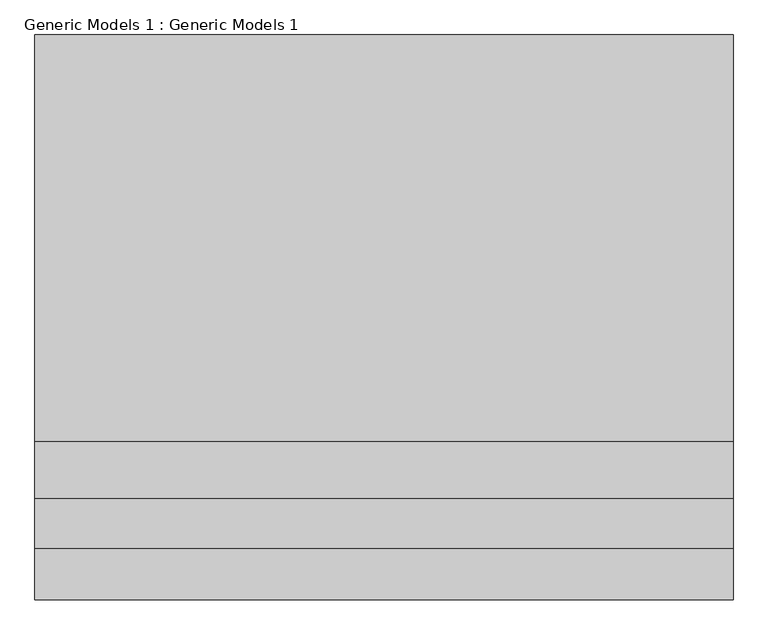
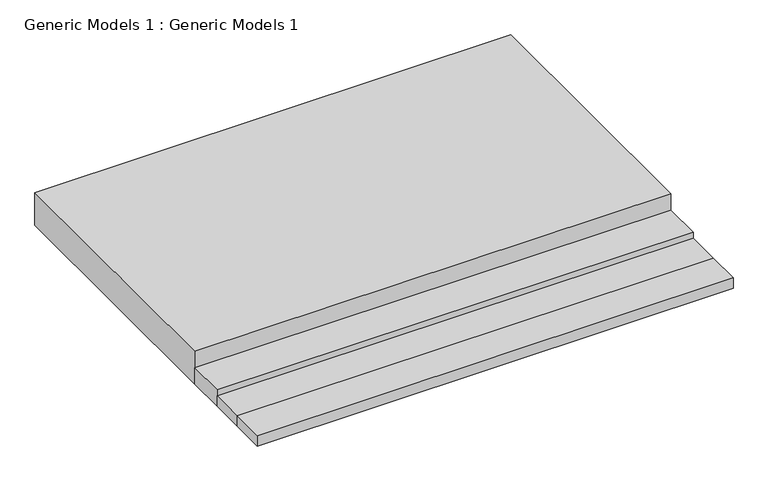
"""IFC4 building model written with IfcOpenShell, lengths in millimetres: proxy geometry, Generic Models 1 : Generic Models 1."""

from ifc_helpers import new_model, si_unit, origin, origin_with_axes, place, context, project, spatial, polyline, outline, extrude, source, transform, mapped, element, save


def generic_models_1_generic_models_1_0112e005(model_context):
    return source(origin(), model_context, "Body", "SweptSolid", [
        extrude(outline(polyline([(1409.039189, -14328.5451307), (-2781.960811, -14328.5451307), (-2781.960811, -14023.7451307), (1409.039189, -14023.7451307), (1409.039189, -14328.5451307)])), origin_with_axes(), (0.0, 0.0, 1.0), 97.9433853),
        extrude(outline(polyline([(1409.039189, -14023.7451307), (-2781.960811, -14023.7451307), (-2781.960811, -13718.9451307), (1409.039189, -13718.9451307), (1409.039189, -14023.7451307)])), origin_with_axes(), (0.0, 0.0, 1.0), 97.9433853),
        extrude(outline(polyline([(1409.039189, -13718.9451307), (-2781.960811, -13718.9451307), (-2781.960811, -13376.4602599), (1409.039189, -13376.4602599), (1409.039189, -13718.9451307)])), origin_with_axes(), (0.0, 0.0, 1.0), 152.4),
        extrude(outline(polyline([(1409.039189, -10938.0602599), (1409.039189, -13376.4602599), (-2781.960811, -13376.4602599), (-2781.960811, -10938.0602599), (1409.039189, -10938.0602599)])), origin_with_axes(), (0.0, 0.0, 1.0), 304.8),
    ])


if __name__ == "__main__":
    model = new_model("IFC4")
    model_context = context("Model", 3, world=origin())
    ifc_project = project(units=[si_unit("LENGTHUNIT", "METRE", prefix="MILLI")], contexts=[model_context])
    site = spatial("IfcSite", under=ifc_project)
    building = spatial("IfcBuilding", under=site)
    placement = place(None, origin())
    generic_models_1_generic_models_1_shape = generic_models_1_generic_models_1_0112e005(model_context)
    element("IfcBuildingElementProxy", 1, Name="Generic Models 1 : Generic Models 1", ObjectType="Generic Models 1 : Generic Models 1", at=placement, inside=building, context=model_context, shape_type="MappedRepresentation", body=[
        mapped(generic_models_1_generic_models_1_shape, transform((0.0, 0.0, 0.0), x_axis=(1.0, 0.0, 0.0), y_axis=(0.0, 1.0, 0.0), z_axis=(0.0, 0.0, 1.0))),
    ])
    save(model, "model.ifc")
